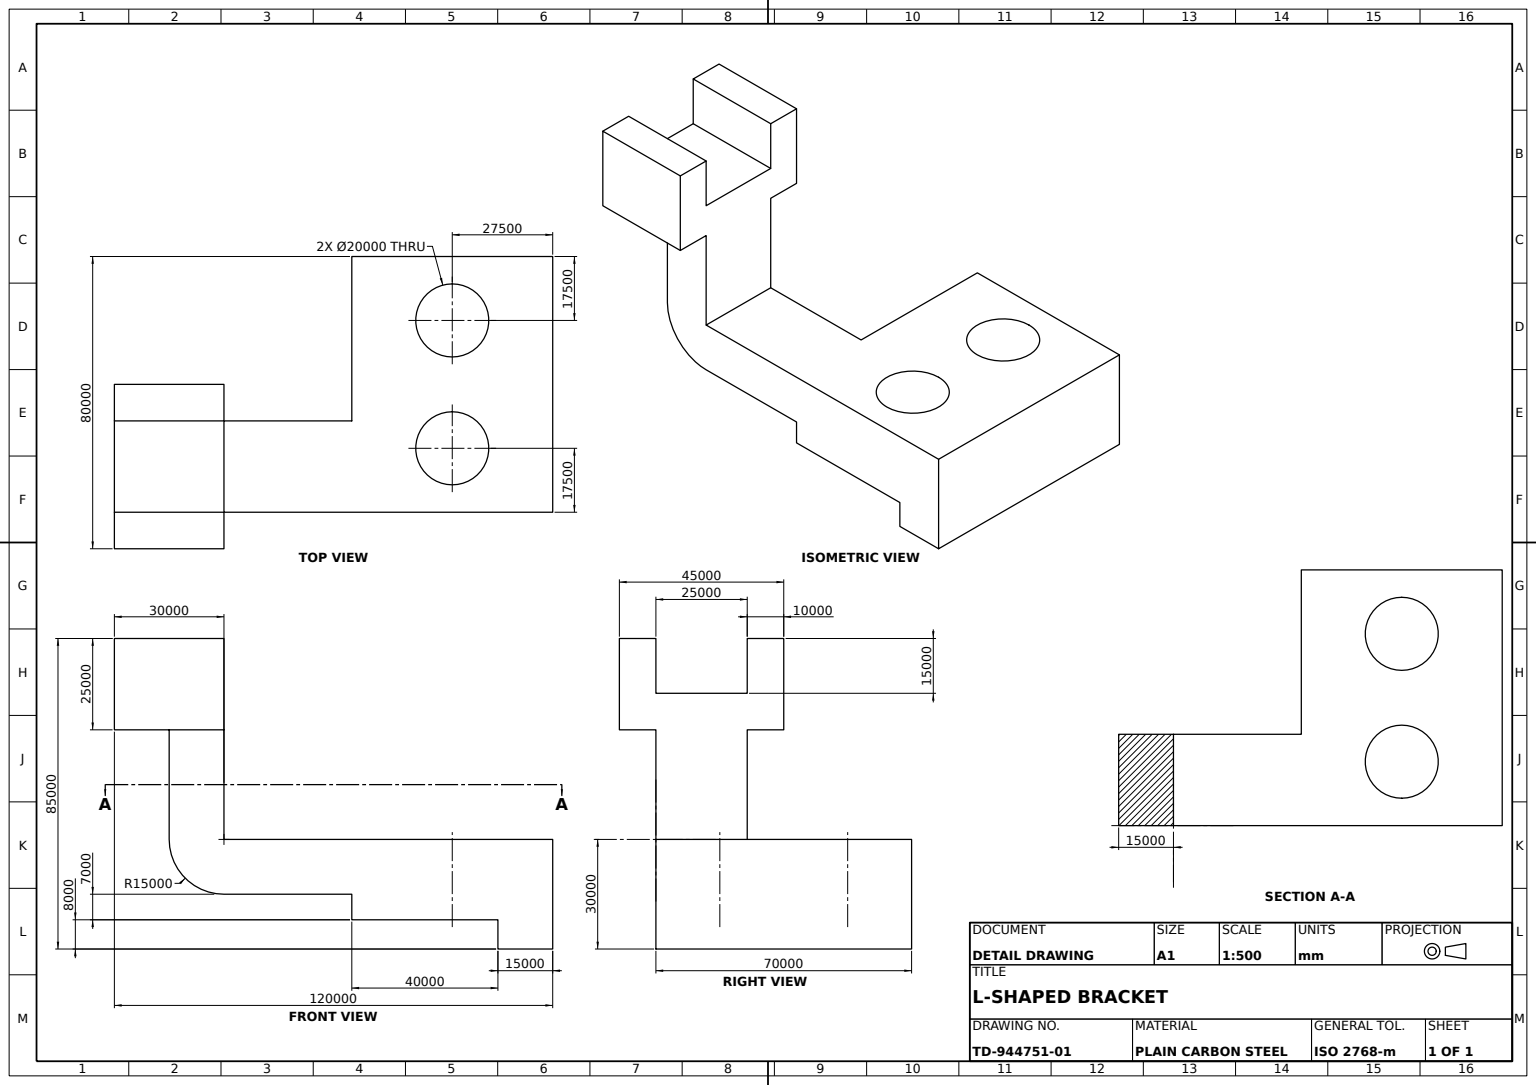
SolidWorks part; units mm, degrees
material "Plain Carbon Steel"
ref_plane "Front Plane" through (0, 0, 0) normal (0, 0, 1) x (1, 0, 0)
ref_plane "Top Plane" through (0, 0, 0) normal (0, 1, 0) x (1, 0, 0)
ref_plane "Right Plane" through (0, 0, 0) normal (1, 0, 0) x (0, 0, -1)
sketch "Base Plate Profile Sketch" plane through (0, 0, 0) normal (0, 0, 1) x (1, 0, 0)
  line L0 (27500, -15000) -> (12500, -15000)
  line L1 (-27500, 15000) -> (27500, 15000)
  line L2 (-27500, 14474.1098) -> (-27500, -7000)
  line L3 (12500, -15000) -> (27500, -15000)
  line L4 (27500, 15000) -> (27500, -15000)
  line L5 (-27500, 14474.1098) -> (-27500, 15000)
  line L7 (12500, -15000) -> (12500, -7000)
  line L8 (12500, -7000) -> (-27500, -7000)
  line L9 (-27500, -7000) -> (-27500, -718.5576)
  line L10 (-27500, 14474.1098) -> (-27500, -718.5576)
  point P0 (0, 0)
  dimension "D1" = 30000
  dimension "D2" = 27500
  dimension "D3" = 15000
  dimension "D4" = 40000
  dimension "D5" = 7000
  dimension "D6" = 15000
  dimension "D7" = 14281.4424
  dimension "D8" = 29474.1098
extrude "Base Plate" add sketch "Base Plate Profile Sketch" along normal mid plane 70000 contours L8 L7 L0 L4 L1 L5 L2
sketch "Upright Arm Sketch" plane through (0, 15000, 0) normal (0, 1, 0) x (1, 0, 0)
  line L1 (-27500, -35000) -> (-77500, -35000)
  line L2 (-27500, -35000) -> (-27500, -10000)
  line L3 (-27500, -10000) -> (-77500, -10000)
  line L4 (-77500, -35000) -> (-77500, -10000)
  dimension "D1" = 25000
  dimension "D2" = 50000
extrude "Upright Arm" add sketch "Upright Arm Sketch" against normal blind 15000
sketch "Upright Extension Sketch" plane through (0, 15000, 0) normal (0, 1, 0) x (1, 0, 0)
  line L0 (-27500, -10000) -> (-77500, -10000) construction
  line L1 (-77500, -35000) -> (-62500, -35000)
  line L2 (-77500, -35000) -> (-77500, -10000)
  line L3 (-77500, -10000) -> (-62500, -10000)
  line L4 (-62500, -35000) -> (-62500, -10000)
  dimension "D1" = 15000
extrude "Upright Extension" add sketch "Upright Extension Sketch" along normal blind 30000
fillet "Bend Fillet R15" radius 15000 1 edges at (-77500, 0, 22500)
sketch "Fork Head Sketch" plane through (-62500, 0, 0) normal (1, 0, 0) x (0, 0, -1)
  line L0 (-10000, 45000) -> (-35000, 45000) construction
  line L1 (0, 45000) -> (-45000, 45000)
  line L2 (0, 45000) -> (0, 70000)
  line L4 (-45000, 45000) -> (-45000, 70000)
  line L7 (-10000, 15000) -> (-10000, 45000) construction
  line L8 (0, 70000) -> (-10000, 70000)
  line L9 (-10000, 70000) -> (-10000, 55000)
  line L10 (-10000, 55000) -> (-35000, 55000)
  line L11 (-35000, 55000) -> (-35000, 70000)
  line L12 (-35000, 70000) -> (-45000, 70000)
  dimension "D1" = 45000
  dimension "D2" = 25000
  dimension "D3" = 0
  dimension "D4" = 10000
  dimension "D5" = 15000
  dimension "D6" = 10000
  dimension "D7" = 25000
  dimension "D8" = 10000
extrude "Fork Head" add sketch "Fork Head Sketch" against normal blind 30000
sketch "Mounting Holes Sketch" plane through (0, 15000, 0) normal (0, 1, 0) x (1, 0, 0)
  line L0 (0, 0) -> (0, -17500) construction
  line L1 (0, 0) -> (0, 17500) construction
  circle A0 centre (0, 17500) radius 10000
  circle A1 centre (0, -17500) radius 10000
  dimension "D3" = 20000
  dimension "D4" = 20000
  dimension "D1" = 17500
  dimension "D2" = 17500
extrude "Mounting Holes 2xØ20" cut sketch "Mounting Holes Sketch" against normal blind 30000
